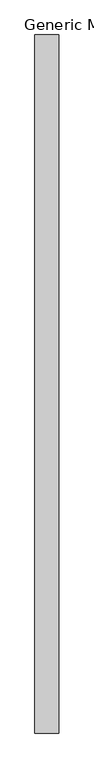
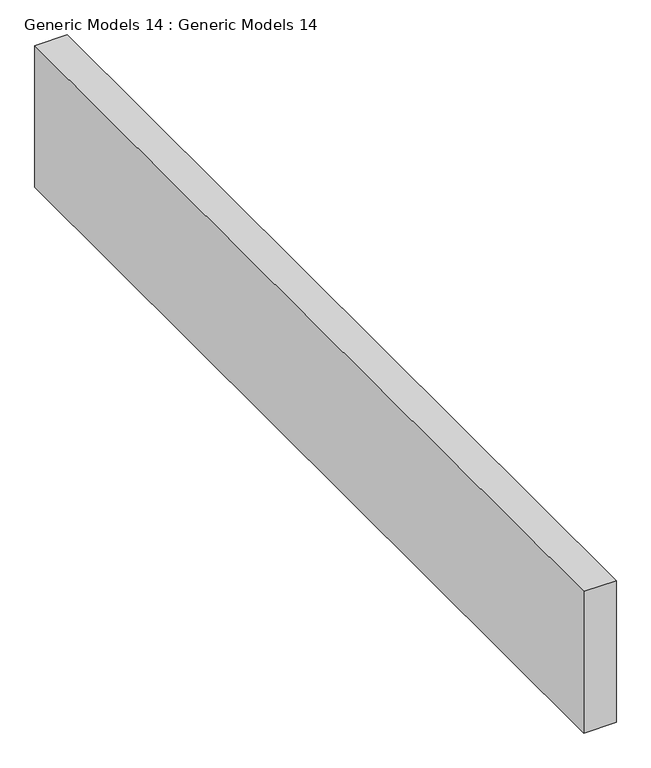
"""IFC4 building model written with IfcOpenShell, lengths in millimetres: proxy geometry, Generic Models 14 : Generic Models 14."""

from ifc_helpers import new_model, si_unit, frame, origin, place, context, project, spatial, polyline, outline, extrude, source, transform, mapped, element, save


def generic_models_14_generic_models_14_41b81b58(model_context):
    return source(origin(), model_context, "Body", "SweptSolid", [
        extrude(outline(polyline([(-6249.8280307, 3771.0498903), (-6249.8280307, 8253.6385461), (-6097.4280307, 8253.6385461), (-6097.4280307, 3771.0498903), (-6249.8280307, 3771.0498903)])), frame((0.0, 0.0, 6299.2), z_axis=(0.0, 0.0, 1.0), x_axis=(1.0, 0.0, 0.0)), (0.0, 0.0, 1.0), 706.2700341),
    ])


if __name__ == "__main__":
    model = new_model("IFC4")
    model_context = context("Model", 3, world=origin())
    ifc_project = project(units=[si_unit("LENGTHUNIT", "METRE", prefix="MILLI")], contexts=[model_context])
    site = spatial("IfcSite", under=ifc_project)
    building = spatial("IfcBuilding", under=site)
    placement = place(None, origin())
    generic_models_14_generic_models_14_shape = generic_models_14_generic_models_14_41b81b58(model_context)
    element("IfcBuildingElementProxy", 1, Name="Generic Models 14 : Generic Models 14", ObjectType="Generic Models 14 : Generic Models 14", at=placement, inside=building, context=model_context, shape_type="MappedRepresentation", body=[
        mapped(generic_models_14_generic_models_14_shape, transform((0.0, 0.0, 0.0), x_axis=(1.0, 0.0, 0.0), y_axis=(0.0, 1.0, 0.0), z_axis=(0.0, 0.0, 1.0))),
    ])
    save(model, "model.ifc")

# Revit data of these elements
# Element 1 (IfcBuildingElementProxy, "Generic Models 14 : Generic Models 14")
#   Materials on its faces: "chocolate brown"
# Materials
#   "chocolate brown": class "Generic", colour RGB 120 120 120, transparency 0, Cost = 0
